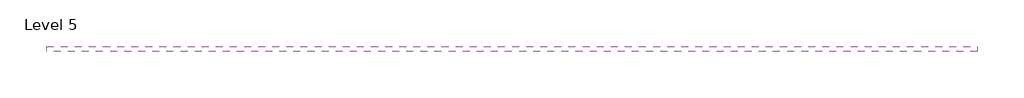
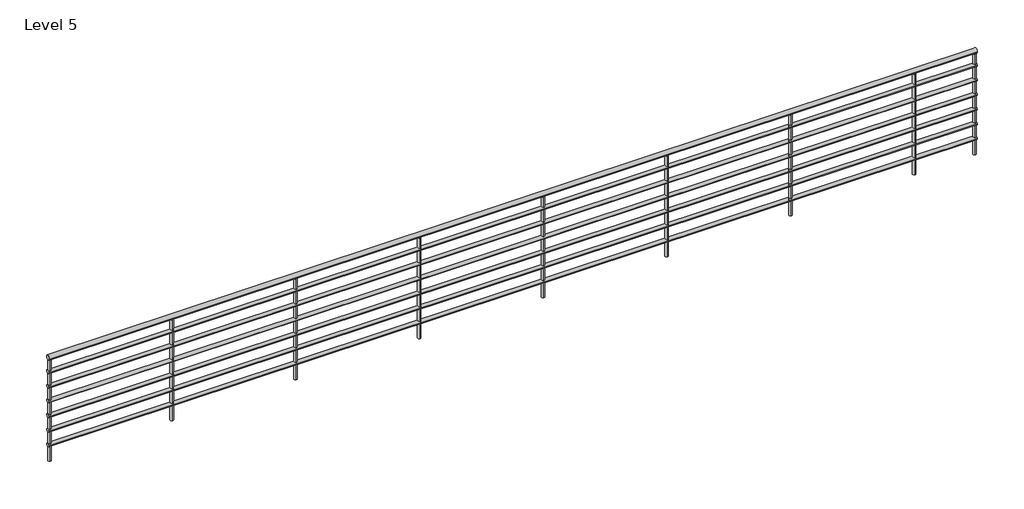
# One storey: 1 railing.
"""IFC4 building model written with IfcOpenShell, lengths in millimetres."""

from ifc_helpers import new_model, si_unit, point, frame, frame_2d, origin, place, context, project, spatial, circle_curve, trimmed, segment, composite_curve, outline, extrude, element, save

model = new_model("IFC4")

# Units and contexts
model_context = context("Model", 3, world=origin())
ifc_project = project(units=[si_unit("LENGTHUNIT", "METRE", prefix="MILLI")], contexts=[model_context])

# Site, building, storey
site = spatial("IfcSite", under=ifc_project)
building = spatial("IfcBuilding", under=site)
storey = spatial("IfcBuildingStorey", under=building, Name="Level 5", Elevation=4000.0)

# Railing
placement = place(None, origin())
element("IfcRailing", 1, ObjectType="900mm Pipe", at=placement, inside=storey, context=model_context, shape_type="SweptSolid", body=[
    extrude(outline(composite_curve([segment(trimmed(circle_curve(frame_2d((-9516.4007969, 12906.410379)), 20.0), [point((-9536.4007969, 12906.410379))], [point((-9496.4007969, 12906.410379))], False, "CARTESIAN"), True, "CONTINUOUS"), segment(trimmed(circle_curve(frame_2d((-9516.4007969, 12906.410379)), 20.0), [point((-9496.4007969, 12906.410379))], [point((-9536.4007969, 12906.410379))], False, "CARTESIAN"), True, "CONTINUOUS")], self_intersect=False)), frame((-8994.8535954, 0.0, 0.0), z_axis=(1.0, 0.0, 0.0), x_axis=(0.0, 1.0, 0.0)), (0.0, 0.0, 1.0), 7500.0),
    extrude(outline(composite_curve([segment(trimmed(circle_curve(frame_2d((-9516.4007969, 12786.410379)), 15.0), [point((-9501.4007969, 12786.410379))], [point((-9531.4007969, 12786.410379))], False, "CARTESIAN"), True, "CONTINUOUS"), segment(trimmed(circle_curve(frame_2d((-9516.4007969, 12786.410379)), 15.0), [point((-9531.4007969, 12786.410379))], [point((-9501.4007969, 12786.410379))], False, "CARTESIAN"), True, "CONTINUOUS")], self_intersect=False)), frame((-8994.8535954, 0.0, 0.0), z_axis=(1.0, 0.0, 0.0), x_axis=(0.0, 1.0, 0.0)), (0.0, 0.0, 1.0), 7500.0),
    extrude(outline(composite_curve([segment(trimmed(circle_curve(frame_2d((-9516.4007969, 12661.410379)), 15.0), [point((-9501.4007969, 12661.410379))], [point((-9531.4007969, 12661.410379))], False, "CARTESIAN"), True, "CONTINUOUS"), segment(trimmed(circle_curve(frame_2d((-9516.4007969, 12661.410379)), 15.0), [point((-9531.4007969, 12661.410379))], [point((-9501.4007969, 12661.410379))], False, "CARTESIAN"), True, "CONTINUOUS")], self_intersect=False)), frame((-8994.8535954, 0.0, 0.0), z_axis=(1.0, 0.0, 0.0), x_axis=(0.0, 1.0, 0.0)), (0.0, 0.0, 1.0), 7500.0),
    extrude(outline(composite_curve([segment(trimmed(circle_curve(frame_2d((-9516.4007969, 12536.410379)), 15.0), [point((-9501.4007969, 12536.410379))], [point((-9531.4007969, 12536.410379))], False, "CARTESIAN"), True, "CONTINUOUS"), segment(trimmed(circle_curve(frame_2d((-9516.4007969, 12536.410379)), 15.0), [point((-9531.4007969, 12536.410379))], [point((-9501.4007969, 12536.410379))], False, "CARTESIAN"), True, "CONTINUOUS")], self_intersect=False)), frame((-8994.8535954, 0.0, 0.0), z_axis=(1.0, 0.0, 0.0), x_axis=(0.0, 1.0, 0.0)), (0.0, 0.0, 1.0), 7500.0),
    extrude(outline(composite_curve([segment(trimmed(circle_curve(frame_2d((-9516.4007969, 12411.410379)), 15.0), [point((-9501.4007969, 12411.410379))], [point((-9531.4007969, 12411.410379))], False, "CARTESIAN"), True, "CONTINUOUS"), segment(trimmed(circle_curve(frame_2d((-9516.4007969, 12411.410379)), 15.0), [point((-9531.4007969, 12411.410379))], [point((-9501.4007969, 12411.410379))], False, "CARTESIAN"), True, "CONTINUOUS")], self_intersect=False)), frame((-8994.8535954, 0.0, 0.0), z_axis=(1.0, 0.0, 0.0), x_axis=(0.0, 1.0, 0.0)), (0.0, 0.0, 1.0), 7500.0),
    extrude(outline(composite_curve([segment(trimmed(circle_curve(frame_2d((-9516.4007969, 12286.410379)), 15.0), [point((-9501.4007969, 12286.410379))], [point((-9531.4007969, 12286.410379))], False, "CARTESIAN"), True, "CONTINUOUS"), segment(trimmed(circle_curve(frame_2d((-9516.4007969, 12286.410379)), 15.0), [point((-9531.4007969, 12286.410379))], [point((-9501.4007969, 12286.410379))], False, "CARTESIAN"), True, "CONTINUOUS")], self_intersect=False)), frame((-8994.8535954, 0.0, 0.0), z_axis=(1.0, 0.0, 0.0), x_axis=(0.0, 1.0, 0.0)), (0.0, 0.0, 1.0), 7500.0),
    extrude(outline(composite_curve([segment(trimmed(circle_curve(frame_2d((-9516.4007969, 12161.410379)), 15.0), [point((-9501.4007969, 12161.410379))], [point((-9531.4007969, 12161.410379))], False, "CARTESIAN"), True, "CONTINUOUS"), segment(trimmed(circle_curve(frame_2d((-9516.4007969, 12161.410379)), 15.0), [point((-9531.4007969, 12161.410379))], [point((-9501.4007969, 12161.410379))], False, "CARTESIAN"), True, "CONTINUOUS")], self_intersect=False)), frame((-8994.8535954, 0.0, 0.0), z_axis=(1.0, 0.0, 0.0), x_axis=(0.0, 1.0, 0.0)), (0.0, 0.0, 1.0), 7500.0),
    extrude(outline(composite_curve([segment(trimmed(circle_curve(frame_2d((-1994.8535954, -9516.4007969)), 12.5), [point((-1994.8535954, -9503.9007969))], [point((-1994.8535954, -9528.9007969))], False, "CARTESIAN"), True, "CONTINUOUS"), segment(trimmed(circle_curve(frame_2d((-1994.8535954, -9516.4007969)), 12.5), [point((-1994.8535954, -9528.9007969))], [point((-1994.8535954, -9503.9007969))], False, "CARTESIAN"), True, "CONTINUOUS")], self_intersect=False)), frame((0.0, 0.0, 12026.410379), z_axis=(0.0, 0.0, 1.0), x_axis=(1.0, 0.0, 0.0)), (0.0, 0.0, 1.0), 860.0),
    extrude(outline(composite_curve([segment(trimmed(circle_curve(frame_2d((-2994.8535954, -9516.4007969)), 12.5), [point((-2994.8535954, -9503.9007969))], [point((-2994.8535954, -9528.9007969))], False, "CARTESIAN"), True, "CONTINUOUS"), segment(trimmed(circle_curve(frame_2d((-2994.8535954, -9516.4007969)), 12.5), [point((-2994.8535954, -9528.9007969))], [point((-2994.8535954, -9503.9007969))], False, "CARTESIAN"), True, "CONTINUOUS")], self_intersect=False)), frame((0.0, 0.0, 12026.410379), z_axis=(0.0, 0.0, 1.0), x_axis=(1.0, 0.0, 0.0)), (0.0, 0.0, 1.0), 860.0),
    extrude(outline(composite_curve([segment(trimmed(circle_curve(frame_2d((-3994.8535954, -9516.4007969)), 12.5), [point((-3994.8535954, -9503.9007969))], [point((-3994.8535954, -9528.9007969))], False, "CARTESIAN"), True, "CONTINUOUS"), segment(trimmed(circle_curve(frame_2d((-3994.8535954, -9516.4007969)), 12.5), [point((-3994.8535954, -9528.9007969))], [point((-3994.8535954, -9503.9007969))], False, "CARTESIAN"), True, "CONTINUOUS")], self_intersect=False)), frame((0.0, 0.0, 12026.410379), z_axis=(0.0, 0.0, 1.0), x_axis=(1.0, 0.0, 0.0)), (0.0, 0.0, 1.0), 860.0),
    extrude(outline(composite_curve([segment(trimmed(circle_curve(frame_2d((-4994.8535954, -9516.4007969)), 12.5), [point((-4994.8535954, -9503.9007969))], [point((-4994.8535954, -9528.9007969))], False, "CARTESIAN"), True, "CONTINUOUS"), segment(trimmed(circle_curve(frame_2d((-4994.8535954, -9516.4007969)), 12.5), [point((-4994.8535954, -9528.9007969))], [point((-4994.8535954, -9503.9007969))], False, "CARTESIAN"), True, "CONTINUOUS")], self_intersect=False)), frame((0.0, 0.0, 12026.410379), z_axis=(0.0, 0.0, 1.0), x_axis=(1.0, 0.0, 0.0)), (0.0, 0.0, 1.0), 860.0),
    extrude(outline(composite_curve([segment(trimmed(circle_curve(frame_2d((-5994.8535954, -9516.4007969)), 12.5), [point((-5994.8535954, -9503.9007969))], [point((-5994.8535954, -9528.9007969))], False, "CARTESIAN"), True, "CONTINUOUS"), segment(trimmed(circle_curve(frame_2d((-5994.8535954, -9516.4007969)), 12.5), [point((-5994.8535954, -9528.9007969))], [point((-5994.8535954, -9503.9007969))], False, "CARTESIAN"), True, "CONTINUOUS")], self_intersect=False)), frame((0.0, 0.0, 12026.410379), z_axis=(0.0, 0.0, 1.0), x_axis=(1.0, 0.0, 0.0)), (0.0, 0.0, 1.0), 860.0),
    extrude(outline(composite_curve([segment(trimmed(circle_curve(frame_2d((-6994.8535954, -9516.4007969)), 12.5), [point((-6994.8535954, -9503.9007969))], [point((-6994.8535954, -9528.9007969))], False, "CARTESIAN"), True, "CONTINUOUS"), segment(trimmed(circle_curve(frame_2d((-6994.8535954, -9516.4007969)), 12.5), [point((-6994.8535954, -9528.9007969))], [point((-6994.8535954, -9503.9007969))], False, "CARTESIAN"), True, "CONTINUOUS")], self_intersect=False)), frame((0.0, 0.0, 12026.410379), z_axis=(0.0, 0.0, 1.0), x_axis=(1.0, 0.0, 0.0)), (0.0, 0.0, 1.0), 860.0),
    extrude(outline(composite_curve([segment(trimmed(circle_curve(frame_2d((-7994.8535954, -9516.4007969)), 12.5), [point((-7994.8535954, -9503.9007969))], [point((-7994.8535954, -9528.9007969))], False, "CARTESIAN"), True, "CONTINUOUS"), segment(trimmed(circle_curve(frame_2d((-7994.8535954, -9516.4007969)), 12.5), [point((-7994.8535954, -9528.9007969))], [point((-7994.8535954, -9503.9007969))], False, "CARTESIAN"), True, "CONTINUOUS")], self_intersect=False)), frame((0.0, 0.0, 12026.410379), z_axis=(0.0, 0.0, 1.0), x_axis=(1.0, 0.0, 0.0)), (0.0, 0.0, 1.0), 860.0),
    extrude(outline(composite_curve([segment(trimmed(circle_curve(frame_2d((-1507.3535954, -9516.4007969)), 12.5), [point((-1507.3535954, -9503.9007969))], [point((-1507.3535954, -9528.9007969))], False, "CARTESIAN"), True, "CONTINUOUS"), segment(trimmed(circle_curve(frame_2d((-1507.3535954, -9516.4007969)), 12.5), [point((-1507.3535954, -9528.9007969))], [point((-1507.3535954, -9503.9007969))], False, "CARTESIAN"), True, "CONTINUOUS")], self_intersect=False)), frame((0.0, 0.0, 12026.410379), z_axis=(0.0, 0.0, 1.0), x_axis=(1.0, 0.0, 0.0)), (0.0, 0.0, 1.0), 860.0),
    extrude(outline(composite_curve([segment(trimmed(circle_curve(frame_2d((-8982.3535954, -9516.4007969)), 12.5), [point((-8982.3535954, -9503.9007969))], [point((-8982.3535954, -9528.9007969))], False, "CARTESIAN"), True, "CONTINUOUS"), segment(trimmed(circle_curve(frame_2d((-8982.3535954, -9516.4007969)), 12.5), [point((-8982.3535954, -9528.9007969))], [point((-8982.3535954, -9503.9007969))], False, "CARTESIAN"), True, "CONTINUOUS")], self_intersect=False)), frame((0.0, 0.0, 12026.410379), z_axis=(0.0, 0.0, 1.0), x_axis=(1.0, 0.0, 0.0)), (0.0, 0.0, 1.0), 860.0),
])

save(model, "model.ifc")

# Revit data of these elements
# Type "900mm Pipe"
#   built-in parameter 1008612 = 0.019685 (stored number, unit not read)
#   built-in parameter 1008611 = 0.0984252 (stored number, unit not read)
#   built-in parameter 1008609 = 6.56168 (stored number, unit not read)
#   built-in parameter 1008604 = 0.19685 (stored number, unit not read)
#   built-in parameter 1008603 = 0.164042 (stored number, unit not read)
#   Railing Height = 2' - 11.43307"
#   built-in parameter 1008630 = 2
#   built-in parameter 1008610 = 2
#   built-in parameter 1008605 = 1
#   built-in parameter 1008618 = M_Baluster - Round : 25mm
# Element 1 (IfcRailing, "900mm Pipe")
#   built-in parameter 1008621 = 26.3334 (stored number, unit not read)
#   Phase Created = New Construction
